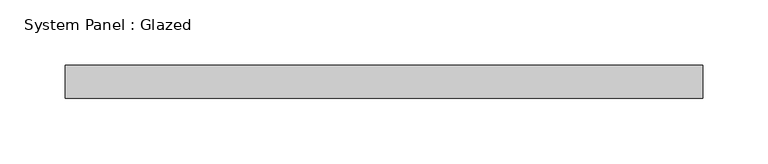
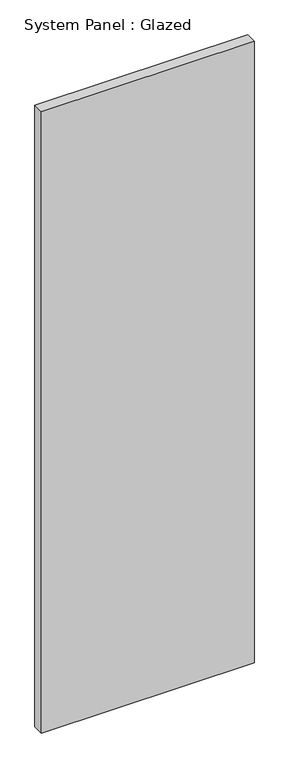
"""IFC4 building model written with IfcOpenShell, lengths in millimetres: plate geometry, System Panel : Glazed."""

from ifc_helpers import new_model, si_unit, origin, origin_with_axes, place, context, project, spatial, polyline, outline, extrude, source, transform, mapped, element, save


def system_panel_glazed_6e344361(model_context):
    return source(origin(), model_context, "Body", "SweptSolid", [
        extrude(outline(polyline([(244.475, 19.05), (-244.475, 19.05), (-244.475, 44.45), (244.475, 44.45), (244.475, 19.05)])), origin_with_axes(), (0.0, 0.0, 1.0), 1509.844519),
    ])


if __name__ == "__main__":
    model = new_model("IFC4")
    model_context = context("Model", 3, world=origin())
    ifc_project = project(units=[si_unit("LENGTHUNIT", "METRE", prefix="MILLI")], contexts=[model_context])
    site = spatial("IfcSite", under=ifc_project)
    building = spatial("IfcBuilding", under=site)
    placement = place(None, origin())
    system_panel_glazed_shape = system_panel_glazed_6e344361(model_context)
    element("IfcPlate", 1, ObjectType="System Panel : Glazed", at=placement, inside=building, context=model_context, shape_type="MappedRepresentation", body=[
        mapped(system_panel_glazed_shape, transform((0.0, 0.0, 0.0), x_axis=(1.0, 0.0, 0.0), y_axis=(0.0, 1.0, 0.0), z_axis=(0.0, 0.0, 1.0))),
    ])
    save(model, "model.ifc")

# Revit data of these elements
# Type "System Panel : Glazed"
#   Construction Type Id = "GSP4R"
#   Analytic Construction = "1/8 in Pilkington single glazing"
#   Visual Light Transmittance = 0.9
#   Solar Heat Gain Coefficient = 0.86
#   Heat Transfer Coefficient (U) = 1.18115 BTU/(h·ft²·°F)
#   Define Thermal Properties by = 1
# Element 1 (IfcPlate, "System Panel : Glazed")
#   Materials on its faces: "Glass"
# Materials
#   "Glass": class "Glass", colour RGB 0 128 192, transparency 0.75, Description = "Soda Lime Glass", Cost = 0
